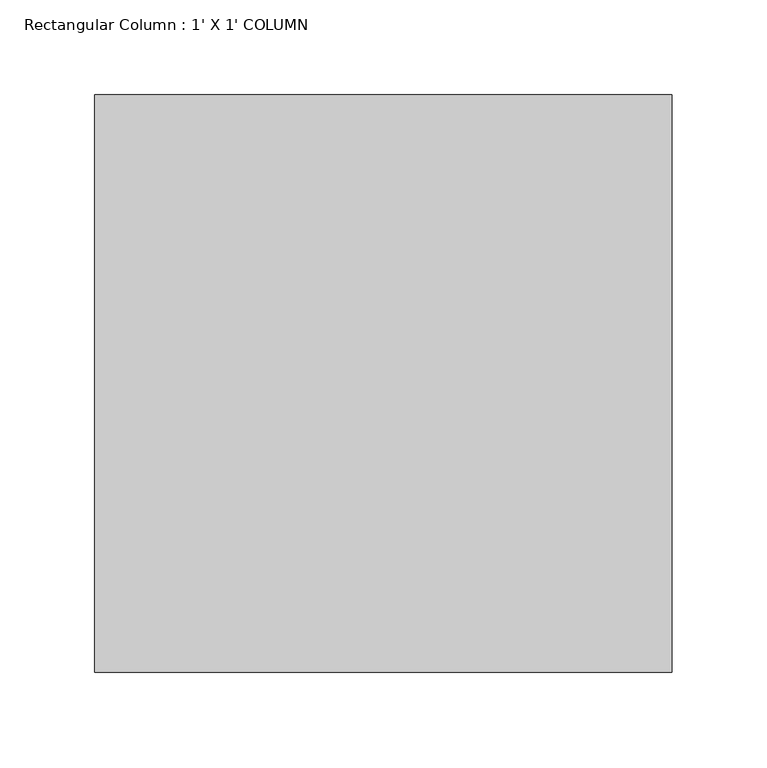
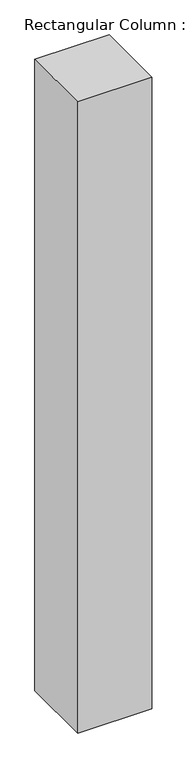
"""IFC4 building model written with IfcOpenShell, lengths in millimetres: column geometry, Rectangular Column : 1' X 1' COLUMN."""

from ifc_helpers import new_model, si_unit, frame, origin, place, context, project, spatial, polyline, outline, extrude, source, transform, mapped, element, save


def rectangular_column_1_x_1_column_3bfae6ee(model_context):
    return source(origin(), model_context, "Body", "SweptSolid", [
        extrude(outline(polyline([(152.4, 152.4), (152.4, -152.4), (-152.4, -152.4), (-152.4, 152.4), (152.4, 152.4)])), frame((0.0, 0.0, 12496.8), z_axis=(0.0, 0.0, 1.0), x_axis=(1.0, 0.0, 0.0)), (0.0, 0.0, 1.0), 2743.2),
    ])


if __name__ == "__main__":
    model = new_model("IFC4")
    model_context = context("Model", 3, world=origin())
    ifc_project = project(units=[si_unit("LENGTHUNIT", "METRE", prefix="MILLI")], contexts=[model_context])
    site = spatial("IfcSite", under=ifc_project)
    building = spatial("IfcBuilding", under=site)
    placement = place(None, origin())
    rectangular_column_1_x_1_column_shape = rectangular_column_1_x_1_column_3bfae6ee(model_context)
    element("IfcColumn", 1, ObjectType="Rectangular Column : 1' X 1' COLUMN", at=placement, inside=building, context=model_context, shape_type="MappedRepresentation", body=[
        mapped(rectangular_column_1_x_1_column_shape, transform((0.0, 0.0, 0.0), x_axis=(1.0, 0.0, 0.0), y_axis=(0.0, 1.0, 0.0), z_axis=(0.0, 0.0, 1.0))),
    ])
    save(model, "model.ifc")

# Revit data of these elements
# Type "Rectangular Column : 1' X 1' COLUMN"
#   Assembly Code = "B1010200"
#   Depth = 1' - 0"
#   Offset Base = 0' - 0"
#   Offset Top = 0' - 0"
#   Width = 1' - 0"
#   Material = SAND BEIGE PAINT
# Element 1 (IfcColumn, "Rectangular Column : 1' X 1' COLUMN")
#   Materials on its faces: "SAND BEIGE PAINT"
# Materials
#   "SAND BEIGE PAINT": class "Generic", colour RGB 120 120 120, transparency 0, Cost = 0
